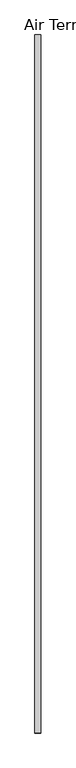
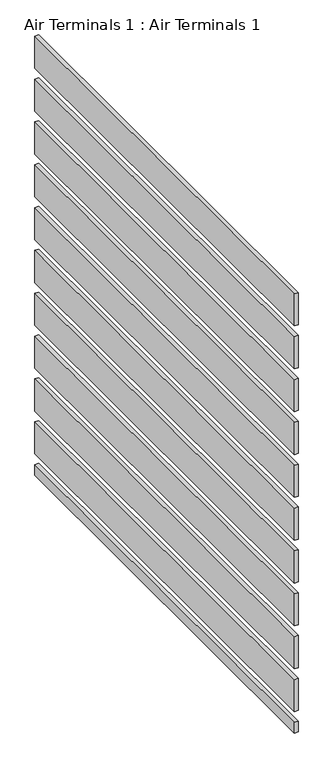
"""IFC4 building model written with IfcOpenShell, lengths in millimetres: air terminal geometry, Air Terminals 1 : Air Terminals 1."""

from ifc_helpers import new_model, si_unit, frame, origin, place, context, project, spatial, polyline, outline, extrude, source, transform, mapped, element, save


def air_terminals_1_air_terminals_1_05a11ed2(model_context):
    return source(origin(), model_context, "Body", "SweptSolid", [
        extrude(outline(polyline([(6782.7574466, -5938.1831508), (6782.7574466, -8960.7831508), (6757.3574466, -8960.7831508), (6757.3574466, -5938.1831508), (6782.7574466, -5938.1831508)])), frame((0.0, 0.0, 3048.0), z_axis=(0.0, 0.0, 1.0), x_axis=(1.0, 0.0, 0.0)), (0.0, 0.0, 1.0), 76.2),
        extrude(outline(polyline([(6782.7574466, -5938.1831508), (6782.7574466, -8960.7831508), (6757.3574466, -8960.7831508), (6757.3574466, -5938.1831508), (6782.7574466, -5938.1831508)])), frame((0.0, 0.0, 5943.6), z_axis=(0.0, 0.0, 1.0), x_axis=(1.0, 0.0, 0.0)), (0.0, 0.0, 1.0), 228.6),
        extrude(outline(polyline([(6782.7574466, -5938.1831508), (6782.7574466, -8960.7831508), (6757.3574466, -8960.7831508), (6757.3574466, -5938.1831508), (6782.7574466, -5938.1831508)])), frame((0.0, 0.0, 5638.8), z_axis=(0.0, 0.0, 1.0), x_axis=(1.0, 0.0, 0.0)), (0.0, 0.0, 1.0), 228.6),
        extrude(outline(polyline([(6782.7574466, -5938.1831508), (6782.7574466, -8960.7831508), (6757.3574466, -8960.7831508), (6757.3574466, -5938.1831508), (6782.7574466, -5938.1831508)])), frame((0.0, 0.0, 5334.0), z_axis=(0.0, 0.0, 1.0), x_axis=(1.0, 0.0, 0.0)), (0.0, 0.0, 1.0), 228.6),
        extrude(outline(polyline([(6782.7574466, -5938.1831508), (6782.7574466, -8960.7831508), (6757.3574466, -8960.7831508), (6757.3574466, -5938.1831508), (6782.7574466, -5938.1831508)])), frame((0.0, 0.0, 5029.2), z_axis=(0.0, 0.0, 1.0), x_axis=(1.0, 0.0, 0.0)), (0.0, 0.0, 1.0), 228.6),
        extrude(outline(polyline([(6782.7574466, -5938.1831508), (6782.7574466, -8960.7831508), (6757.3574466, -8960.7831508), (6757.3574466, -5938.1831508), (6782.7574466, -5938.1831508)])), frame((0.0, 0.0, 4724.4), z_axis=(0.0, 0.0, 1.0), x_axis=(1.0, 0.0, 0.0)), (0.0, 0.0, 1.0), 228.6),
        extrude(outline(polyline([(6782.7574466, -5938.1831508), (6782.7574466, -8960.7831508), (6757.3574466, -8960.7831508), (6757.3574466, -5938.1831508), (6782.7574466, -5938.1831508)])), frame((0.0, 0.0, 4419.6), z_axis=(0.0, 0.0, 1.0), x_axis=(1.0, 0.0, 0.0)), (0.0, 0.0, 1.0), 228.6),
        extrude(outline(polyline([(6782.7574466, -5938.1831508), (6782.7574466, -8960.7831508), (6757.3574466, -8960.7831508), (6757.3574466, -5938.1831508), (6782.7574466, -5938.1831508)])), frame((0.0, 0.0, 4114.8), z_axis=(0.0, 0.0, 1.0), x_axis=(1.0, 0.0, 0.0)), (0.0, 0.0, 1.0), 228.6),
        extrude(outline(polyline([(6782.7574466, -5938.1831508), (6782.7574466, -8960.7831508), (6757.3574466, -8960.7831508), (6757.3574466, -5938.1831508), (6782.7574466, -5938.1831508)])), frame((0.0, 0.0, 3810.0), z_axis=(0.0, 0.0, 1.0), x_axis=(1.0, 0.0, 0.0)), (0.0, 0.0, 1.0), 228.6),
        extrude(outline(polyline([(6782.7574466, -5938.1831508), (6782.7574466, -8960.7831508), (6757.3574466, -8960.7831508), (6757.3574466, -5938.1831508), (6782.7574466, -5938.1831508)])), frame((0.0, 0.0, 3505.2), z_axis=(0.0, 0.0, 1.0), x_axis=(1.0, 0.0, 0.0)), (0.0, 0.0, 1.0), 228.6),
        extrude(outline(polyline([(6782.7574466, -5938.1831508), (6782.7574466, -8960.7831508), (6757.3574466, -8960.7831508), (6757.3574466, -5938.1831508), (6782.7574466, -5938.1831508)])), frame((0.0, 0.0, 3200.4), z_axis=(0.0, 0.0, 1.0), x_axis=(1.0, 0.0, 0.0)), (0.0, 0.0, 1.0), 228.6),
    ])


if __name__ == "__main__":
    model = new_model("IFC4")
    model_context = context("Model", 3, world=origin())
    ifc_project = project(units=[si_unit("LENGTHUNIT", "METRE", prefix="MILLI")], contexts=[model_context])
    site = spatial("IfcSite", under=ifc_project)
    building = spatial("IfcBuilding", under=site)
    placement = place(None, origin())
    air_terminals_1_air_terminals_1_shape = air_terminals_1_air_terminals_1_05a11ed2(model_context)
    element("IfcAirTerminal", 1, ObjectType="Air Terminals 1 : Air Terminals 1", at=placement, inside=building, context=model_context, shape_type="MappedRepresentation", body=[
        mapped(air_terminals_1_air_terminals_1_shape, transform((0.0, 0.0, 0.0), x_axis=(1.0, 0.0, 0.0), y_axis=(0.0, 1.0, 0.0), z_axis=(0.0, 0.0, 1.0))),
    ])
    save(model, "model.ifc")
